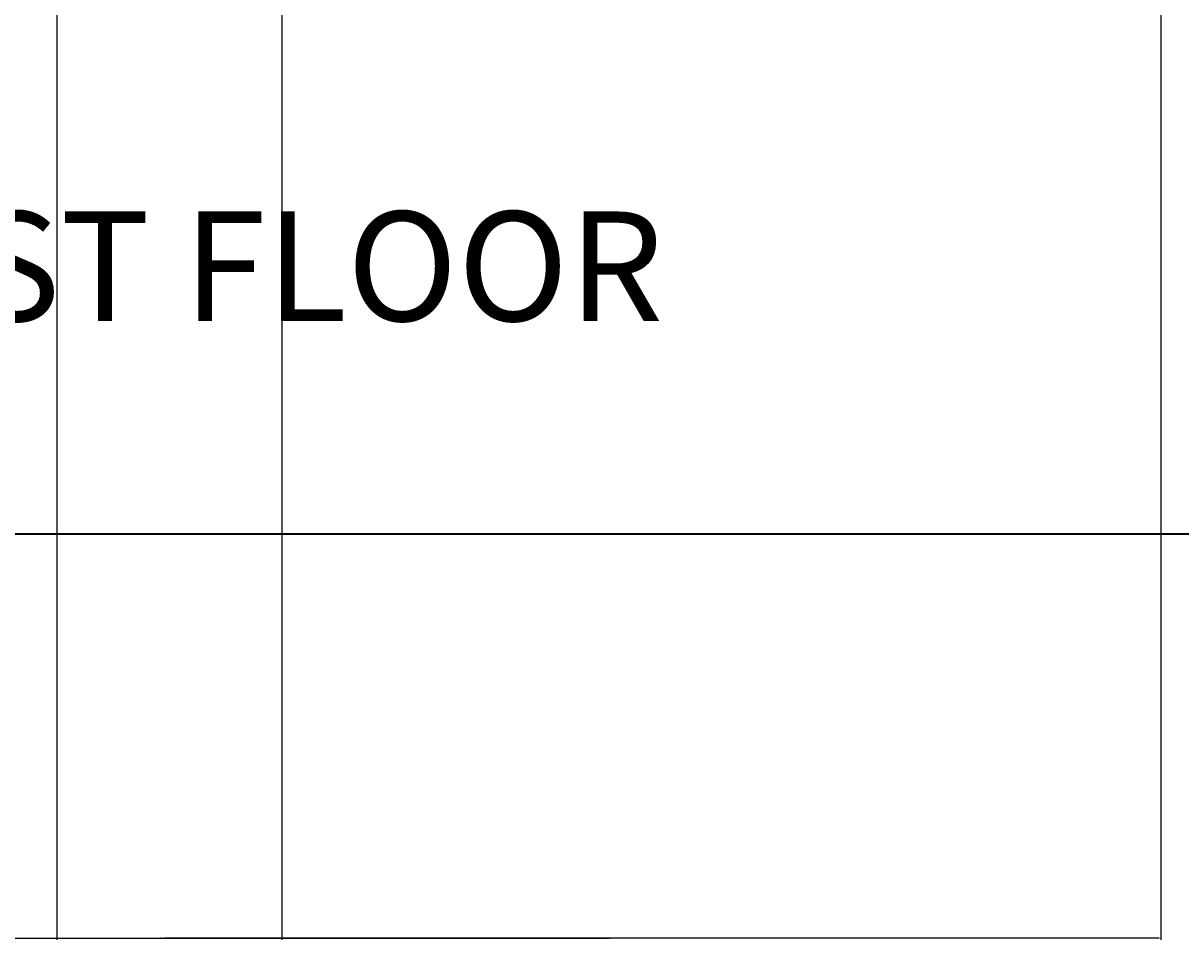
# Model space of a CAD drawing. Units: feet. Extents: x 2100 to 2836, y 2433 to 3396.
# Tile 3 of 12: x 2616 to 2743, y 2433 to 2533. Entities that reach past the tile are written whole.
import ezdxf

# ---------------------------------------------------------------- set-up
doc = ezdxf.new("R2010")
doc.units = ezdxf.units.FT
for name, color, linetype, lineweight in [('A-ANNO-DIMS', 2, 'Continuous', 18), ('A-ANNO-TITL', 7, 'Continuous', 25), ('A-ANNO-TTLB', 7, 'Continuous', 35)]:
    doc.layers.add(name, color=color, linetype=linetype, lineweight=lineweight)
doc.styles.get("Standard").update_dxf_attribs({"font": 'arial.ttf'})
doc.dimstyles.get("Standard").update_dxf_attribs({"dimtxt": 0.18, "dimasz": 0.18, "dimexe": 0.18, "dimexo": 0.0625, "dimgap": 0.09, "dimtad": 0, "dimtih": 1, "dimtoh": 1, "dimdec": 4, "dimzin": 0, "dimdsep": 46, "dimtxsty": 'Standard', "dimcen": 0.09, "dimadec": 0, "dimazin": 0, "dimtfac": 1, "dimtdec": 4, "dimtofl": 0, "dimtmove": 0, "dimatfit": 3, "dimfxl": 1, "dimtolj": 1, "dimtzin": 0, "dimarcsym": 0})

# ---------------------------------------------------------------- blocks, each defined once
blk = doc.blocks.new('*D42')
at = {"layer": 'A-ANNO-DIMS', "color": 0, "lineweight": -2, "transparency": 16777216}
for p, q in [((2521.95, 2537.69), (2521.95, 2433.01)), ((2740.95, 2537.69), (2740.95, 2433.01)), ((2522.13, 2433.19), (2631.16, 2433.19)), ((2740.77, 2433.19), (2631.74, 2433.19))]:
    blk.add_line(p, q, dxfattribs=at)
at = {"layer": 'A-ANNO-DIMS', "color": 0, "transparency": 16777216}
for points in [[(2522.13, 2433.22), (2522.13, 2433.16), (2521.95, 2433.19)], [(2740.77, 2433.22), (2740.77, 2433.16), (2740.95, 2433.19)]]:
    blk.add_solid(points, dxfattribs=at)
at = {"layer": 'Defpoints', "color": 0, "transparency": 16777216}
for p in [(2521.95, 2537.76), (2740.95, 2537.76), (2740.95, 2433.19)]:
    blk.add_point(p, dxfattribs=at)
at = {"layer": 'A-ANNO-DIMS', "color": 0, "transparency": 16777216, "insert": (2631.45, 2433.19), "char_height": 0.18, "attachment_point": 5}
blk.add_mtext('\\A1;219', dxfattribs=at)
blk = doc.blocks.new('*D65')
at = {"layer": 'A-ANNO-DIMS', "color": 0, "lineweight": -2, "transparency": 16777216}
for p, q in [((2619.95, 2624.74), (2619.95, 2433.01)), ((2644.63, 2624.74), (2644.63, 2433.01)), ((2620.13, 2433.19), (2631.83, 2433.19)), ((2644.45, 2433.19), (2632.76, 2433.19))]:
    blk.add_line(p, q, dxfattribs=at)
at = {"layer": 'A-ANNO-DIMS', "color": 0, "transparency": 16777216}
for points in [[(2620.13, 2433.22), (2620.13, 2433.16), (2619.95, 2433.19)], [(2644.45, 2433.22), (2644.45, 2433.16), (2644.63, 2433.19)]]:
    blk.add_solid(points, dxfattribs=at)
at = {"layer": 'Defpoints', "color": 0, "transparency": 16777216}
for p in [(2619.95, 2624.8), (2644.63, 2624.8), (2644.63, 2433.19)]:
    blk.add_point(p, dxfattribs=at)
at = {"layer": 'A-ANNO-DIMS', "color": 0, "transparency": 16777216, "insert": (2632.29, 2433.19), "char_height": 0.18, "attachment_point": 5}
blk.add_mtext('\\A1;24.686', dxfattribs=at)
blk = doc.blocks.new('*D66')
at = {"layer": 'A-ANNO-DIMS', "color": 0, "lineweight": -2, "transparency": 16777216}
for p, q in [((2619.95, 2584.74), (2619.95, 2433.01)), ((2740.95, 2584.74), (2740.95, 2433.01)), ((2620.13, 2433.19), (2680.18, 2433.19)), ((2740.77, 2433.19), (2680.71, 2433.19))]:
    blk.add_line(p, q, dxfattribs=at)
at = {"layer": 'A-ANNO-DIMS', "color": 0, "transparency": 16777216}
for points in [[(2620.13, 2433.22), (2620.13, 2433.16), (2619.95, 2433.19)], [(2740.77, 2433.22), (2740.77, 2433.16), (2740.95, 2433.19)]]:
    blk.add_solid(points, dxfattribs=at)
at = {"layer": 'Defpoints', "color": 0, "transparency": 16777216}
for p in [(2619.95, 2584.8), (2740.95, 2584.8), (2740.95, 2433.19)]:
    blk.add_point(p, dxfattribs=at)
at = {"layer": 'A-ANNO-DIMS', "color": 0, "transparency": 16777216, "insert": (2680.45, 2433.19), "char_height": 0.18, "attachment_point": 5}
blk.add_mtext('\\A1;121', dxfattribs=at)

msp = doc.modelspace()

# ---------------------------------------------------------------- linework, layer by layer
at = {"layer": 'A-ANNO-TTLB'}
msp.add_lwpolyline([(2144.0848, 3351.6245), (2791.0561, 3351.6245), (2791.0561, 2477.4373), (2144.0848, 2477.4373)], close=True, dxfattribs=at)

# ---------------------------------------------------------------- texts
at = {"layer": 'A-ANNO-TITL'}
msp.add_text('FIRST FLOOR', height=12, dxfattribs=at).set_placement((2586.3598, 2500.7808))

# ---------------------------------------------------------------- dimensions: what is measured, and where the dimension line sits
at = {"layer": 'A-ANNO-DIMS'}
for base, p1, p2, override, picture, middle in [((2644.6339, 2433.1873), (2619.9476, 2624.8031), (2644.6339, 2624.8031), {"dimdec": 3, "dimlfac": 1, "dimrnd": 0, "dimzin": 0, "dimdsep": 46, "dimlunit": 2}, '*D65', (2632.2907, 2433.1873)), ((2740.9476, 2433.1873), (2619.9476, 2584.8031), (2740.9476, 2584.8031), {"dimdec": 0, "dimlfac": 1, "dimrnd": 0, "dimzin": 0, "dimdsep": 46, "dimlunit": 2}, '*D66', (2680.4476, 2433.1873)), ((2740.9476, 2433.1873), (2521.9476, 2537.755), (2740.9476, 2537.755), {"dimdec": 0, "dimlfac": 1, "dimrnd": 0, "dimzin": 0, "dimdsep": 46, "dimlunit": 2}, '*D42', (2631.4476, 2433.1873))]:
    dim = msp.add_linear_dim(base=base, p1=p1, p2=p2, dimstyle='Standard', override=override, dxfattribs=at)
    dim.commit()
    dim.dimension.update_dxf_attribs({"geometry": picture, "text_midpoint": middle})

doc.saveas('drawing.dxf')
